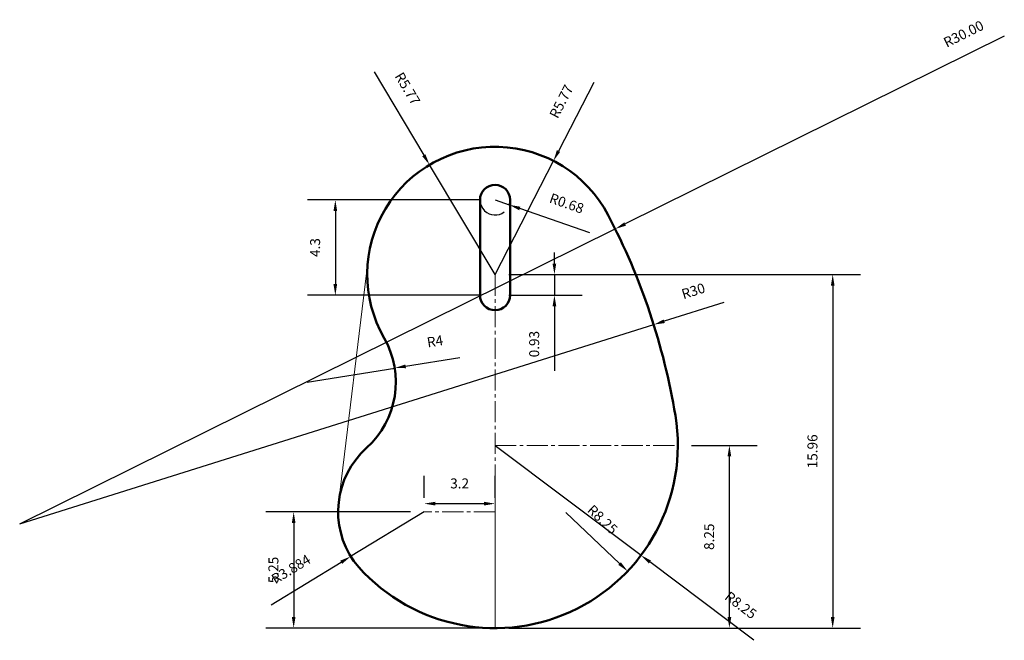
# Model space of a CAD drawing. Units: millimetres. Extents: x 3105.9 to 3150.3, y 1656.4 to 1684.4.
import ezdxf

# ---------------------------------------------------------------- set-up
doc = ezdxf.new("R2010")
doc.units = ezdxf.units.MM
doc.linetypes.add('CENTER2', pattern=[28.575, 19.05, -3.175, 3.175, -3.175])
for name, color, linetype, lineweight in [('M-CNTR', 1, 'CENTER2', 18), ('M-CONS', 8, 'Continuous', 18), ('M-DIMS', 2, 'Continuous', 25), ('M-OUTL', 7, 'Continuous', 50)]:
    doc.layers.add(name, color=color, linetype=linetype, lineweight=lineweight)
doc.styles.get("Standard").update_dxf_attribs({"font": 'arial.ttf'})
doc.dimstyles.new('ISO-25', dxfattribs={"dimtxt": 0.45, "dimasz": 0.5, "dimexe": 1.25, "dimexo": 0.625, "dimtad": 1, "dimdsep": 46, "dimtxsty": 'Standard', "dimcen": 2.5, "dimadec": 0, "dimazin": 0, "dimtfac": 1, "dimtmove": 0, "dimatfit": 3, "dimfxl": 1, "dimarcsym": 0})

# ---------------------------------------------------------------- blocks, each defined once
blk = doc.blocks.new('*D1')
at = {"layer": 'Defpoints', "color": 0, "transparency": 16777216}
for p in [(3127.358, 1665.175), (3133.342, 1659.496)]:
    blk.add_point(p, dxfattribs=at)
at = {"layer": 'M-DIMS', "color": 0, "lineweight": -2, "transparency": 16777216}
blk.add_line((3130.547, 1662.148), (3132.979, 1659.84), dxfattribs=at)
at = {"layer": 'M-DIMS', "color": 0, "transparency": 16777216}
blk.add_solid([(3133.036, 1659.901), (3132.922, 1659.78), (3133.342, 1659.496)], dxfattribs=at)
at = {"layer": 'M-DIMS', "color": 0, "transparency": 16777216, "insert": (3132.17, 1661.786), "char_height": 0.45, "attachment_point": 5, "rotation": 316.4941}
blk.add_mtext('R8.25', dxfattribs=at)
blk = doc.blocks.new('*D2')
at = {"layer": 'Defpoints', "color": 0, "transparency": 16777216}
for p in [(3127.358, 1672.885), (3127.358, 1656.925), (3142.6, 1656.925)]:
    blk.add_point(p, dxfattribs=at)
at = {"layer": 'M-DIMS', "color": 0, "lineweight": -2, "transparency": 16777216}
for p, q in [((3127.983, 1672.885), (3143.85, 1672.885)), ((3142.6, 1672.385), (3142.6, 1657.425)), ((3127.983, 1656.925), (3143.85, 1656.925))]:
    blk.add_line(p, q, dxfattribs=at)
at = {"layer": 'M-DIMS', "color": 0, "transparency": 16777216}
for points in [[(3142.517, 1672.385), (3142.683, 1672.385), (3142.6, 1672.885)], [(3142.517, 1657.425), (3142.683, 1657.425), (3142.6, 1656.925)]]:
    blk.add_solid(points, dxfattribs=at)
at = {"layer": 'M-DIMS', "color": 0, "transparency": 16777216, "insert": (3141.745, 1664.905), "char_height": 0.45, "attachment_point": 5, "rotation": 90}
blk.add_mtext('15.96', dxfattribs=at)
blk = doc.blocks.new('*D3')
at = {"layer": 'Defpoints', "color": 0, "transparency": 16777216}
for p in [(3135.608, 1665.175), (3137.936, 1665.175), (3127.358, 1656.925)]:
    blk.add_point(p, dxfattribs=at)
at = {"layer": 'M-DIMS', "color": 0, "lineweight": -2, "transparency": 16777216}
for p, q in [((3136.233, 1665.175), (3139.186, 1665.175)), ((3137.936, 1657.425), (3137.936, 1664.675)), ((3127.983, 1656.925), (3139.186, 1656.925))]:
    blk.add_line(p, q, dxfattribs=at)
at = {"layer": 'M-DIMS', "color": 0, "transparency": 16777216}
for points in [[(3137.853, 1664.675), (3138.02, 1664.675), (3137.936, 1665.175)], [(3137.853, 1657.425), (3138.02, 1657.425), (3137.936, 1656.925)]]:
    blk.add_solid(points, dxfattribs=at)
at = {"layer": 'M-DIMS', "color": 0, "transparency": 16777216, "insert": (3137.081, 1661.05), "char_height": 0.45, "attachment_point": 5, "rotation": 90}
blk.add_mtext('8.25', dxfattribs=at)
blk = doc.blocks.new('*D4')
at = {"layer": 'Defpoints', "color": 0, "transparency": 16777216}
for p in [(3124.158, 1662.175), (3118.266, 1656.925), (3127.358, 1656.925)]:
    blk.add_point(p, dxfattribs=at)
at = {"layer": 'M-DIMS', "color": 0, "lineweight": -2, "transparency": 16777216}
for p, q in [((3123.533, 1662.175), (3117.016, 1662.175)), ((3118.266, 1661.675), (3118.266, 1657.425)), ((3126.733, 1656.925), (3117.016, 1656.925))]:
    blk.add_line(p, q, dxfattribs=at)
at = {"layer": 'M-DIMS', "color": 0, "transparency": 16777216}
for points in [[(3118.183, 1661.675), (3118.349, 1661.675), (3118.266, 1662.175)], [(3118.183, 1657.425), (3118.349, 1657.425), (3118.266, 1656.925)]]:
    blk.add_solid(points, dxfattribs=at)
at = {"layer": 'M-DIMS', "color": 0, "transparency": 16777216, "insert": (3117.411, 1659.55), "char_height": 0.45, "attachment_point": 5, "rotation": 90}
blk.add_mtext('5.25', dxfattribs=at)
blk = doc.blocks.new('*D5')
at = {"layer": 'Defpoints', "color": 0, "transparency": 16777216}
for p in [(3127.358, 1662.544), (3124.158, 1662.175), (3127.358, 1662.175)]:
    blk.add_point(p, dxfattribs=at)
at = {"layer": 'M-DIMS', "color": 0, "lineweight": -2, "transparency": 16777216}
for p, q in [((3124.158, 1662.8), (3124.158, 1663.794)), ((3127.358, 1662.8), (3127.358, 1663.794)), ((3124.658, 1662.544), (3126.858, 1662.544))]:
    blk.add_line(p, q, dxfattribs=at)
at = {"layer": 'M-DIMS', "color": 0, "transparency": 16777216}
for points in [[(3124.658, 1662.628), (3124.658, 1662.461), (3124.158, 1662.544)], [(3126.858, 1662.628), (3126.858, 1662.461), (3127.358, 1662.544)]]:
    blk.add_solid(points, dxfattribs=at)
at = {"layer": 'M-DIMS', "color": 0, "transparency": 16777216, "insert": (3125.758, 1663.399), "char_height": 0.45, "attachment_point": 5}
blk.add_mtext('3.2', dxfattribs=at)
blk = doc.blocks.new('*D6')
at = {"layer": 'Defpoints', "color": 0, "transparency": 16777216}
for p in [(3134.519, 1670.627), (3105.898, 1661.635)]:
    blk.add_point(p, dxfattribs=at)
at = {"layer": 'M-DIMS', "color": 0, "lineweight": -2, "transparency": 16777216}
for p, q in [((3137.69, 1671.623), (3134.996, 1670.777)), ((3105.898, 1661.635), (3134.519, 1670.627))]:
    blk.add_line(p, q, dxfattribs=at)
at = {"layer": 'M-DIMS', "color": 0, "transparency": 16777216}
blk.add_solid([(3134.971, 1670.856), (3135.021, 1670.697), (3134.519, 1670.627)], dxfattribs=at)
at = {"layer": 'M-DIMS', "color": 0, "transparency": 16777216, "insert": (3136.325, 1672.09), "char_height": 0.45, "attachment_point": 5, "rotation": 17.4405}
blk.add_mtext('R30', dxfattribs=at)
blk = doc.blocks.new('*D7')
at = {"layer": 'Defpoints', "color": 0, "transparency": 16777216}
for p in [(3127.358, 1676.255), (3120.147, 1671.955), (3127.358, 1671.955)]:
    blk.add_point(p, dxfattribs=at)
at = {"layer": 'M-DIMS', "color": 0, "lineweight": -2, "transparency": 16777216}
for p, q in [((3126.733, 1676.255), (3118.897, 1676.255)), ((3120.147, 1675.755), (3120.147, 1672.455)), ((3126.733, 1671.955), (3118.897, 1671.955))]:
    blk.add_line(p, q, dxfattribs=at)
at = {"layer": 'M-DIMS', "color": 0, "transparency": 16777216}
for points in [[(3120.063, 1675.755), (3120.23, 1675.755), (3120.147, 1676.255)], [(3120.063, 1672.455), (3120.23, 1672.455), (3120.147, 1671.955)]]:
    blk.add_solid(points, dxfattribs=at)
at = {"layer": 'M-DIMS', "color": 0, "transparency": 16777216, "insert": (3119.292, 1674.105), "char_height": 0.45, "attachment_point": 5, "rotation": 90}
blk.add_mtext('4.3', dxfattribs=at)
blk = doc.blocks.new('*D8')
at = {"layer": 'Defpoints', "color": 0, "transparency": 16777216}
for p in [(3127.358, 1672.885), (3127.358, 1671.955), (3130.037, 1671.955)]:
    blk.add_point(p, dxfattribs=at)
at = {"layer": 'M-DIMS', "color": 0, "lineweight": -2, "transparency": 16777216}
for p, q in [((3130.037, 1673.385), (3130.037, 1673.885)), ((3127.983, 1672.885), (3131.287, 1672.885)), ((3130.037, 1672.885), (3130.037, 1671.955)), ((3127.983, 1671.955), (3131.287, 1671.955)), ((3130.037, 1671.455), (3130.037, 1668.537))]:
    blk.add_line(p, q, dxfattribs=at)
at = {"layer": 'M-DIMS', "color": 0, "transparency": 16777216}
for points in [[(3129.953, 1673.385), (3130.12, 1673.385), (3130.037, 1672.885)], [(3129.953, 1671.455), (3130.12, 1671.455), (3130.037, 1671.955)]]:
    blk.add_solid(points, dxfattribs=at)
at = {"layer": 'M-DIMS', "color": 0, "transparency": 16777216, "insert": (3129.182, 1669.746), "char_height": 0.45, "attachment_point": 5, "rotation": 90}
blk.add_mtext('0.93', dxfattribs=at)
blk = doc.blocks.new('*D9')
at = {"layer": 'Defpoints', "color": 0, "transparency": 16777216}
for p in [(3129.995, 1678.018), (3127.358, 1672.885)]:
    blk.add_point(p, dxfattribs=at)
at = {"layer": 'M-DIMS', "color": 0, "lineweight": -2, "transparency": 16777216}
for p, q in [((3131.809, 1681.55), (3130.223, 1678.462)), ((3127.358, 1672.885), (3129.995, 1678.018))]:
    blk.add_line(p, q, dxfattribs=at)
at = {"layer": 'M-DIMS', "color": 0, "transparency": 16777216}
blk.add_solid([(3130.149, 1678.501), (3130.297, 1678.424), (3129.995, 1678.018)], dxfattribs=at)
at = {"layer": 'M-DIMS', "color": 0, "transparency": 16777216, "insert": (3130.399, 1680.673), "char_height": 0.45, "attachment_point": 5, "rotation": 62.808}
blk.add_mtext('R5.77', dxfattribs=at)
blk = doc.blocks.new('*D10')
at = {"layer": 'Defpoints', "color": 0, "transparency": 16777216}
for p in [(3127.358, 1676.255), (3128, 1676.033)]:
    blk.add_point(p, dxfattribs=at)
at = {"layer": 'M-DIMS', "color": 0, "lineweight": -2, "transparency": 16777216}
for p, q in [((3127.358, 1676.255), (3128, 1676.033)), ((3131.638, 1674.771), (3128.473, 1675.869))]:
    blk.add_line(p, q, dxfattribs=at)
blk.add_arc((3127.358, 1676.255), 0.68, 340.8769, 307.3384, dxfattribs=at)
at = {"layer": 'M-DIMS', "color": 0, "transparency": 16777216}
blk.add_solid([(3128.5, 1675.948), (3128.445, 1675.79), (3128, 1676.033)], dxfattribs=at)
at = {"layer": 'M-DIMS', "color": 0, "transparency": 16777216, "insert": (3130.572, 1676.046), "char_height": 0.45, "attachment_point": 5, "rotation": 340.8769}
blk.add_mtext('R0.68', dxfattribs=at)
blk = doc.blocks.new('*D11')
at = {"layer": 'Defpoints', "color": 0, "transparency": 16777216}
for p in [(3122.829, 1668.664), (3118.879, 1668.032)]:
    blk.add_point(p, dxfattribs=at)
at = {"layer": 'M-DIMS', "color": 0, "lineweight": -2, "transparency": 16777216}
for p, q in [((3125.765, 1669.133), (3123.322, 1668.743)), ((3118.879, 1668.032), (3122.829, 1668.664))]:
    blk.add_line(p, q, dxfattribs=at)
at = {"layer": 'M-DIMS', "color": 0, "transparency": 16777216}
blk.add_solid([(3123.309, 1668.825), (3123.335, 1668.66), (3122.829, 1668.664)], dxfattribs=at)
at = {"layer": 'M-DIMS', "color": 0, "transparency": 16777216, "insert": (3124.656, 1669.817), "char_height": 0.45, "attachment_point": 5, "rotation": 9.0901}
blk.add_mtext('R4', dxfattribs=at)
blk = doc.blocks.new('*D12')
at = {"layer": 'Defpoints', "color": 0, "transparency": 16777216}
for p in [(3124.4, 1677.839), (3127.358, 1672.885)]:
    blk.add_point(p, dxfattribs=at)
at = {"layer": 'M-DIMS', "color": 0, "lineweight": -2, "transparency": 16777216}
for p, q in [((3121.894, 1682.035), (3124.143, 1678.269)), ((3127.358, 1672.885), (3124.4, 1677.839))]:
    blk.add_line(p, q, dxfattribs=at)
at = {"layer": 'M-DIMS', "color": 0, "transparency": 16777216}
blk.add_solid([(3124.215, 1678.312), (3124.072, 1678.226), (3124.4, 1677.839)], dxfattribs=at)
at = {"layer": 'M-DIMS', "color": 0, "transparency": 16777216, "insert": (3123.358, 1681.25), "char_height": 0.45, "attachment_point": 5, "rotation": 300.8419}
blk.add_mtext('R5.77', dxfattribs=at)
blk = doc.blocks.new('*D13')
at = {"layer": 'Defpoints', "color": 0, "transparency": 16777216}
for p in [(3127.358, 1665.175), (3133.948, 1660.212)]:
    blk.add_point(p, dxfattribs=at)
at = {"layer": 'M-DIMS', "color": 0, "lineweight": -2, "transparency": 16777216}
for p, q in [((3127.358, 1665.175), (3133.948, 1660.212)), ((3139.041, 1656.375), (3134.347, 1659.911))]:
    blk.add_line(p, q, dxfattribs=at)
at = {"layer": 'M-DIMS', "color": 0, "transparency": 16777216}
blk.add_solid([(3134.397, 1659.978), (3134.297, 1659.844), (3133.948, 1660.212)], dxfattribs=at)
at = {"layer": 'M-DIMS', "color": 0, "transparency": 16777216, "insert": (3138.416, 1657.916), "char_height": 0.45, "attachment_point": 5, "rotation": 323.0117}
blk.add_mtext('R8.25', dxfattribs=at)
blk = doc.blocks.new('*D14')
at = {"layer": 'Defpoints', "color": 0, "transparency": 16777216}
for p in [(3124.158, 1662.175), (3120.838, 1660.159)]:
    blk.add_point(p, dxfattribs=at)
at = {"layer": 'M-DIMS', "color": 0, "lineweight": -2, "transparency": 16777216}
for p, q in [((3124.158, 1662.175), (3120.838, 1660.159)), ((3117.251, 1657.98), (3120.411, 1659.899))]:
    blk.add_line(p, q, dxfattribs=at)
at = {"layer": 'M-DIMS', "color": 0, "transparency": 16777216}
blk.add_solid([(3120.367, 1659.97), (3120.454, 1659.828), (3120.838, 1660.159)], dxfattribs=at)
at = {"layer": 'M-DIMS', "color": 0, "transparency": 16777216, "insert": (3118.173, 1659.54), "char_height": 0.45, "attachment_point": 5, "rotation": 31.2771}
blk.add_mtext('R3.884', dxfattribs=at)
blk = doc.blocks.new('*D15')
at = {"layer": 'Defpoints', "color": 0, "transparency": 16777216}
for p in [(3132.783, 1674.947), (3105.898, 1661.635)]:
    blk.add_point(p, dxfattribs=at)
at = {"layer": 'M-DIMS', "color": 0, "lineweight": -2, "transparency": 16777216}
for p, q in [((3150.347, 1683.643), (3133.231, 1675.169)), ((3105.898, 1661.635), (3132.783, 1674.947))]:
    blk.add_line(p, q, dxfattribs=at)
at = {"layer": 'M-DIMS', "color": 0, "transparency": 16777216}
blk.add_solid([(3133.194, 1675.243), (3133.268, 1675.094), (3132.783, 1674.947)], dxfattribs=at)
at = {"layer": 'M-DIMS', "color": 0, "transparency": 16777216, "insert": (3148.535, 1683.7), "char_height": 0.45, "attachment_point": 5, "rotation": 26.3412}
blk.add_mtext('R30.00', dxfattribs=at)

msp = doc.modelspace()

# ---------------------------------------------------------------- linework, layer by layer
at = {"layer": 'M-CNTR', "ltscale": 0.05}
for p, q in [((3127.3578, 1672.8854), (3127.3578, 1656.9255)), ((3127.3578, 1665.1754), (3135.6078, 1665.1754)), ((3127.3578, 1662.1754), (3124.1578, 1662.1754)), ((3127.3578, 1656.9255), (3127.3578, 1662.1754))]:
    msp.add_line(p, q, dxfattribs=at)
at = {"layer": 'M-CONS'}
msp.add_line((3120.2924, 1662.5582), (3121.6282, 1673.5668), dxfattribs=at)
at = {"layer": 'M-OUTL'}
for p, q in [((3126.6778, 1671.9555), (3126.6778, 1676.2555)), ((3128.0378, 1671.9555), (3128.0378, 1676.2555))]:
    msp.add_line(p, q, dxfattribs=at)
for centre, radius, start, end in [((3127.3578, 1672.8854), 5.77, 27.66487, 209.7891), ((3127.3578, 1676.2555), 0.68, 0, 180), ((3105.8978, 1661.6355), 30, 9.36697, 27.66487), ((3127.3578, 1671.9555), 0.68, 180, 0), ((3118.8788, 1668.0316), 4, 312.03276, 29.7891), ((3127.3578, 1665.1754), 8.25, 219.34037, 9.36697), ((3124.1578, 1662.1754), 3.8843, 132.03276, 215.03479)]:
    msp.add_arc(centre, radius, start, end, dxfattribs=at)

# ---------------------------------------------------------------- dimensions: what is measured, and where the dimension line sits
at = {"layer": 'M-DIMS'}
for center, mpoint, override, picture, middle in [((3105.8978, 1661.6355), (3132.7829, 1674.947), {"dimdec": 2, "dimlfac": 1, "dimrnd": 0, "dimzin": 0, "dimdsep": 46, "dimlunit": 2}, '*D15', (3148.9139, 1682.9338)), ((3127.3578, 1672.8854), (3124.3997, 1677.8395), {"dimdec": 2, "dimlfac": 1, "dimrnd": 0, "dimzin": 0, "dimdsep": 46, "dimlunit": 2}, '*D12', (3122.6248, 1680.8119)), ((3127.3578, 1672.8854), (3129.9946, 1678.0178), {"dimclrd": 0, "dimclre": 0, "dimclrt": 0}, '*D9', (3131.1582, 1680.2828)), ((3127.3578, 1665.1754), (3133.3416, 1659.4959), {"dimclrd": 0, "dimclre": 0, "dimclrt": 0}, '*D1', (3131.5817, 1661.1664)), ((3127.3578, 1665.1754), (3133.9476, 1660.2118), {"dimdec": 2, "dimlfac": 1, "dimrnd": 0, "dimzin": 0, "dimdsep": 46, "dimlunit": 2}, '*D13', (3137.9014, 1657.2336))]:
    dim = msp.add_radius_dim(center=center, mpoint=mpoint, dimstyle='ISO-25', override=override, dxfattribs=at)
    dim.commit()
    dim.dimension.update_dxf_attribs({"geometry": picture, "text_midpoint": middle, "dimtype": 164})
for center, mpoint, override, picture, middle in [((3127.3578, 1676.2555), (3128.0003, 1676.0327), {"dimclrd": 0, "dimclre": 0, "dimclrt": 0}, '*D10', (3130.5717, 1676.0458)), ((3105.8978, 1661.6355), (3134.5187, 1670.6269), {"dimclrd": 0, "dimclre": 0, "dimclrt": 0}, '*D6', (3136.325, 1672.0905)), ((3118.8788, 1668.0316), (3122.8286, 1668.6636), {"dimclrd": 0, "dimclre": 0, "dimclrt": 0}, '*D11', (3124.6563, 1669.8168)), ((3124.1578, 1662.1754), (3120.838, 1660.1588), {"dimdec": 3, "dimlfac": 1, "dimrnd": 0, "dimzin": 0, "dimdsep": 46, "dimlunit": 2}, '*D14', (3118.1732, 1659.5403))]:
    dim = msp.add_radius_dim(center=center, mpoint=mpoint, dimstyle='ISO-25', override=override, dxfattribs=at)
    dim.commit()
    dim.dimension.update_dxf_attribs({"geometry": picture, "text_midpoint": middle})
for base, p1, p2, picture, middle in [((3120.1466, 1671.9555), (3127.3578, 1676.2555), (3127.3578, 1671.9555), '*D7', (3119.2917, 1674.1055)), ((3142.5998, 1656.9255), (3127.3578, 1672.8854), (3127.3578, 1656.9255), '*D2', (3141.7451, 1664.9055)), ((3137.9362, 1665.1754), (3127.3578, 1656.9255), (3135.6078, 1665.1754), '*D3', (3137.0815, 1661.0505)), ((3118.2661, 1656.9255), (3124.1578, 1662.1754), (3127.3578, 1656.9255), '*D4', (3117.4114, 1659.5505))]:
    dim = msp.add_linear_dim(base=base, p1=p1, p2=p2, angle=90, dimstyle='ISO-25', override={"dimclrd": 0, "dimclre": 0, "dimclrt": 0}, dxfattribs=at)
    dim.commit()
    dim.dimension.update_dxf_attribs({"geometry": picture, "text_midpoint": middle})
dim = msp.add_aligned_dim(p1=(3127.3578, 1672.8854), p2=(3127.3578, 1671.9555), distance=2.6789, dimstyle='ISO-25', override={"dimclrd": 0, "dimclre": 0, "dimclrt": 0}, dxfattribs=at)
dim.commit()
dim.dimension.update_dxf_attribs({"geometry": '*D8', "text_midpoint": (3129.1818, 1669.746)})
dim = msp.add_linear_dim(base=(3127.3578, 1662.5445), p1=(3124.1578, 1662.1754), p2=(3127.3578, 1662.1754), dimstyle='ISO-25', override={"dimclrd": 0, "dimclre": 0, "dimclrt": 0}, dxfattribs=at)
dim.commit()
dim.dimension.update_dxf_attribs({"geometry": '*D5', "text_midpoint": (3125.7578, 1663.3994)})

doc.saveas('drawing.dxf')
